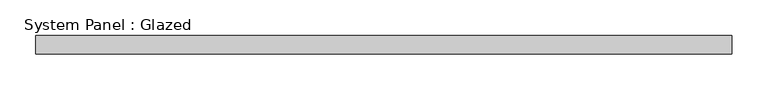
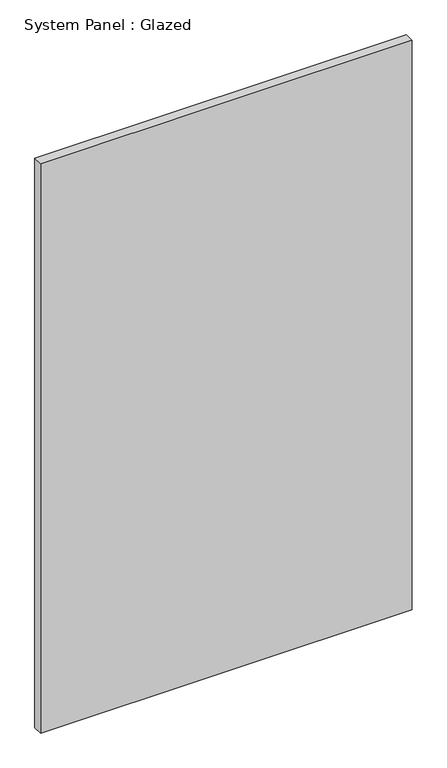
"""IFC4 building model written with IfcOpenShell, lengths in millimetres: plate geometry, System Panel : Glazed."""

from ifc_helpers import new_model, si_unit, origin, origin_with_axes, place, context, project, spatial, polyline, outline, extrude, source, transform, mapped, element, save


def system_panel_glazed_55aea4e3(model_context):
    return source(origin(), model_context, "Body", "SweptSolid", [
        extrude(outline(polyline([(485.775, 19.05), (-485.775, 19.05), (-485.775, 44.45), (485.775, 44.45), (485.775, 19.05)])), origin_with_axes(), (0.0, 0.0, 1.0), 1573.436135),
    ])


if __name__ == "__main__":
    model = new_model("IFC4")
    model_context = context("Model", 3, world=origin())
    ifc_project = project(units=[si_unit("LENGTHUNIT", "METRE", prefix="MILLI")], contexts=[model_context])
    site = spatial("IfcSite", under=ifc_project)
    building = spatial("IfcBuilding", under=site)
    placement = place(None, origin())
    system_panel_glazed_shape = system_panel_glazed_55aea4e3(model_context)
    element("IfcPlate", 1, ObjectType="System Panel : Glazed", at=placement, inside=building, context=model_context, shape_type="MappedRepresentation", body=[
        mapped(system_panel_glazed_shape, transform((0.0, 0.0, 0.0), x_axis=(1.0, 0.0, 0.0), y_axis=(0.0, 1.0, 0.0), z_axis=(0.0, 0.0, 1.0))),
    ])
    save(model, "model.ifc")

# Revit data of these elements
# Type "System Panel : Glazed"
#   Construction Type Id = "GSP4R"
#   Analytic Construction = "1/8 in Pilkington single glazing"
#   Visual Light Transmittance = 0.9
#   Solar Heat Gain Coefficient = 0.86
#   Heat Transfer Coefficient (U) = 1.18115 BTU/(h·ft²·°F)
#   Define Thermal Properties by = 1
# Element 1 (IfcPlate, "System Panel : Glazed")
#   Materials on its faces: "Glass"
# Materials
#   "Glass": class "Glass", colour RGB 0 128 192, transparency 0.75, Description = "Soda Lime Glass", Cost = 0
